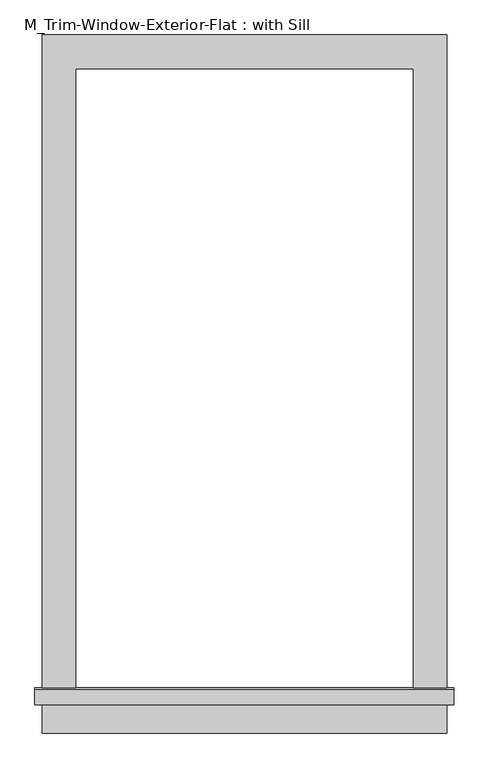
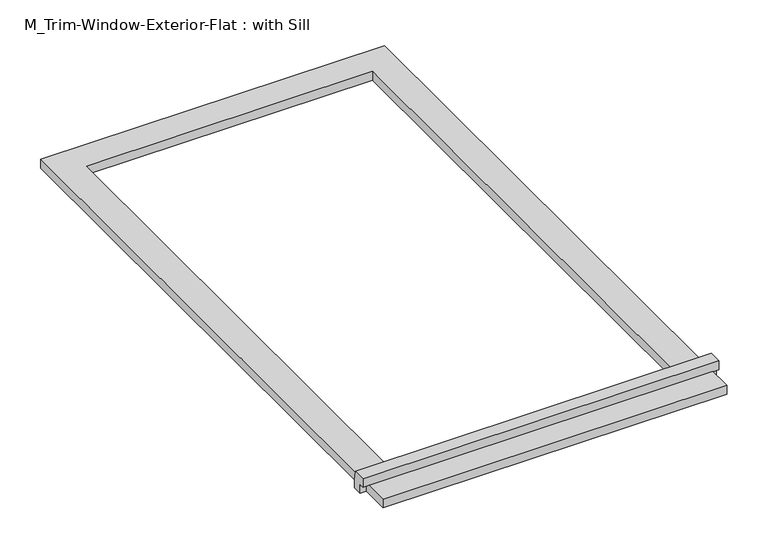
"""IFC4 building model written with IfcOpenShell, lengths in millimetres: proxy geometry, M_Trim-Window-Exterior-Flat : with Sill."""

from ifc_helpers import new_model, si_unit, frame, origin, origin_with_axes, place, context, project, spatial, polyline, outline, extrude, source, transform, mapped, element, save


def m_trim_window_exterior_flat_with_sill_4c9fee41(model_context):
    return source(origin(), model_context, "Body", "SweptSolid", [
        extrude(outline(polyline([(360.0, -1120.4323709), (360.0, -1180.4323709), (-360.0, -1180.4323709), (-360.0, -1120.4323709), (360.0, -1120.4323709)])), origin_with_axes(), (0.0, 0.0, 1.0), 19.05),
        extrude(outline(polyline([(-1130.0, 38.1), (-1102.4580645, 38.1), (-1100.0, 19.05), (-1100.0, 0.0), (-1120.4323709, 0.0), (-1120.4323709, 19.05), (-1130.0, 19.05), (-1130.0, 38.1)])), frame((-372.7, 0.0, 0.0), z_axis=(1.0, 0.0, 0.0), x_axis=(0.0, 1.0, 0.0)), (0.0, 0.0, 1.0), 745.4),
        extrude(outline(polyline([(-360.0, 60.0), (360.0, 60.0), (360.0, -1100.0), (300.0, -1100.0), (300.0, 0.0), (-300.0, 0.0), (-300.0, -1100.0), (-360.0, -1100.0), (-360.0, 60.0)])), origin_with_axes(), (0.0, 0.0, 1.0), 19.05),
    ])


if __name__ == "__main__":
    model = new_model("IFC4")
    model_context = context("Model", 3, world=origin())
    ifc_project = project(units=[si_unit("LENGTHUNIT", "METRE", prefix="MILLI")], contexts=[model_context])
    site = spatial("IfcSite", under=ifc_project)
    building = spatial("IfcBuilding", under=site)
    placement = place(None, origin())
    m_trim_window_exterior_flat_with_sill_shape = m_trim_window_exterior_flat_with_sill_4c9fee41(model_context)
    element("IfcBuildingElementProxy", 1, Name="M_Trim-Window-Exterior-Flat : with Sill", ObjectType="M_Trim-Window-Exterior-Flat : with Sill", at=placement, inside=building, context=model_context, shape_type="MappedRepresentation", body=[
        mapped(m_trim_window_exterior_flat_with_sill_shape, transform((0.0, 0.0, 0.0), x_axis=(1.0, 0.0, 0.0), y_axis=(0.0, 1.0, 0.0), z_axis=(0.0, 0.0, 1.0))),
    ])
    save(model, "model.ifc")

# Revit data of these elements
# Type "M_Trim-Window-Exterior-Flat : with Sill"
#   Trim Width = 0.06 m
#   Trim Thickness_Picture Frame = 0.03 m
#   Trim Thickness_with Sill = 0.01905 m
#   Sill Thickness = 0.03 m
#   Opening Width [instance default] = 0.6 m
#   Opening Height [instance default] = 0.9 m
#   Default Elevation = 1.2 m
#   Sill = yes
#   Picture Frame = no
#   Trim Material [instance default] = none
# Element 1 (IfcBuildingElementProxy, "M_Trim-Window-Exterior-Flat : with Sill")
#   Opening Height = 1.1 m
#   Trim Material = Clad - White
#   Materials on its faces: "Clad - White"
# Materials
#   "Clad - White": class "Wood", colour RGB 242 242 238, transparency 0, Cost = 0
